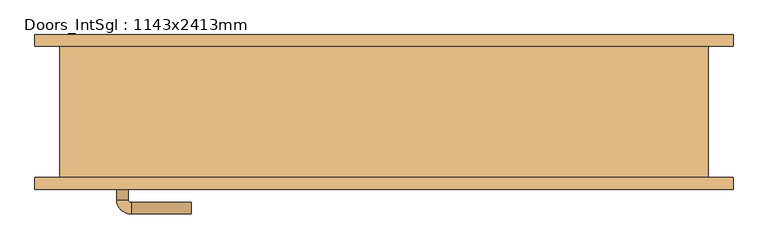
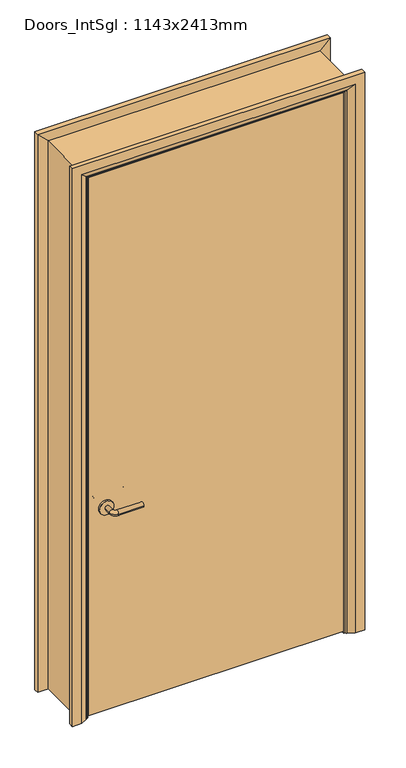
"""IFC4 building model written with IfcOpenShell, lengths in millimetres: door geometry, Doors_IntSgl : 1143x2413mm."""

from ifc_helpers import new_model, si_unit, point, frame, frame_2d, origin, place, context, project, spatial, polyline, circle_curve, ellipse_curve, trimmed, segment, composite_curve, outline, extrude, faceted_brep, source, transform, mapped, element, save
from ifc_brep_helpers import plane_surface, cylinder_surface, revolved_surface, advanced_brep


def doors_intsgl_1143x2413mm_ac4b68bc(model_context):
    return source(origin(), model_context, "Body", "SolidModel", [
        advanced_brep(
        [(-464.5, -68.3, 900.0), (-444.5, -68.3, 900.0), (-464.5, -38.3, 900.0), (-444.5, -38.3, 900.0), (-439.5, -33.3, 900.0), (-439.5, -13.3, 900.0), (-334.5, -13.3, 900.0), (-334.5, -33.3, 900.0)],
        [
            (0, 1, circle_curve(frame((-454.5, -68.3, 900.0), z_axis=(0.0, -1.0, 0.0), x_axis=(1.0, 0.0, 0.0)), 10.0)),
            (1, 0, circle_curve(frame((-454.5, -68.3, 900.0), z_axis=(0.0, -1.0, 0.0), x_axis=(1.0, 0.0, 0.0)), 10.0)),
            (0, 2),
            (2, 3, circle_curve(frame((-454.5, -38.3, 900.0), z_axis=(0.0, -1.0, 0.0), x_axis=(1.0, 0.0, 0.0)), 10.0)),
            (3, 1),
            (3, 2, circle_curve(frame((-454.5, -38.3, 900.0), z_axis=(0.0, -1.0, 0.0), x_axis=(1.0, 0.0, 0.0)), 10.0)),
            (4, 3, circle_curve(frame((-439.5, -38.3, 900.0), z_axis=(0.0, 0.0, 1.0), x_axis=(-1.0, 0.0, 0.0)), 5.0)),
            (2, 5, circle_curve(frame((-439.5, -38.3, 900.0), z_axis=(0.0, 0.0, -1.0), x_axis=(-1.0, 0.0, 0.0)), 25.0)),
            (5, 4, circle_curve(frame((-439.5, -23.3, 900.0), z_axis=(-1.0, 0.0, 0.0), x_axis=(0.0, -1.0, 0.0)), 10.0)),
            (4, 5, circle_curve(frame((-439.5, -23.3, 900.0), z_axis=(-1.0, 0.0, 0.0), x_axis=(0.0, -1.0, 0.0)), 10.0)),
            (6, 7, circle_curve(frame((-334.5, -23.3, 900.0), z_axis=(1.0, 0.0, 0.0), x_axis=(0.0, -1.0, 0.0)), 10.0)),
            (7, 6, circle_curve(frame((-334.5, -23.3, 900.0), z_axis=(1.0, 0.0, 0.0), x_axis=(0.0, -1.0, 0.0)), 10.0)),
            (5, 6),
            (7, 4),
        ],
        [
            plane_surface(frame((-454.5, -68.3, 900.0), z_axis=(0.0, -1.0, 0.0), x_axis=(0.0, 0.0, 1.0))),
            cylinder_surface(frame((-454.5, -68.3, 900.0), z_axis=(0.0, -1.0, 0.0), x_axis=(1.0, 0.0, 0.0)), 10.0),
            revolved_surface(trimmed(ellipse_curve(frame((-454.5, -38.3, 900.0), z_axis=(0.0, -1.0, 0.0), x_axis=(1.0, 0.0, 0.0)), 10.0, 10.0), [point((-464.5, -38.3, 900.0))], [point((-444.5, -38.3, 900.0))], True, "CARTESIAN"), (-439.5, -38.3, 900.0), (0.0, 0.0, -1.0)),
            revolved_surface(trimmed(ellipse_curve(frame((-454.5, -38.3, 900.0), z_axis=(0.0, -1.0, 0.0), x_axis=(1.0, 0.0, 0.0)), 10.0, 10.0), [point((-444.5, -38.3, 900.0))], [point((-464.5, -38.3, 900.0))], True, "CARTESIAN"), (-439.5, -38.3, 900.0), (0.0, 0.0, -1.0)),
            plane_surface(frame((-334.5, -23.3, 900.0), z_axis=(1.0, 0.0, 0.0), x_axis=(0.0, 0.0, 1.0))),
            cylinder_surface(frame((-439.5, -23.3, 900.0), z_axis=(-1.0, 0.0, 0.0), x_axis=(0.0, -1.0, 0.0)), 10.0),
        ],
        [
            (0, [[1, 2]]),
            (1, [[-1, 3, 4, 5]]),
            (1, [[-2, -5, 6, -3]]),
            (2, [[7, -4, 8, 9]]),
            (3, [[-8, -6, -7, 10]]),
            (4, [[11, 12]]),
            (5, [[-9, 13, -12, 14]]),
            (5, [[-10, -14, -11, -13]]),
        ],
    ),
        extrude(outline(composite_curve([segment(trimmed(circle_curve(frame_2d((900.0, -457.0)), 30.0), [point((900.0, -487.0))], [point((900.0, -427.0))], False, "CARTESIAN"), True, "CONTINUOUS"), segment(trimmed(circle_curve(frame_2d((900.0, -457.0)), 30.0), [point((900.0, -427.0))], [point((900.0, -487.0))], False, "CARTESIAN"), True, "CONTINUOUS")], self_intersect=False)), frame((0.0, -76.3, 0.0), z_axis=(0.0, 1.0, 0.0), x_axis=(0.0, 0.0, 1.0)), (0.0, 0.0, 1.0), 8.0),
        advanced_brep(
        [(-464.5, -122.3, 900.0), (-444.5, -122.3, 900.0), (-444.5, -152.3, 900.0), (-464.5, -152.3, 900.0), (-439.5, -157.3, 900.0), (-439.5, -177.3, 900.0), (-334.5, -177.3, 900.0), (-334.5, -157.3, 900.0)],
        [
            (0, 1, circle_curve(frame((-454.5, -122.3, 900.0), z_axis=(0.0, 1.0, 0.0), x_axis=(1.0, 0.0, 0.0)), 10.0)),
            (1, 0, circle_curve(frame((-454.5, -122.3, 900.0), z_axis=(0.0, 1.0, 0.0), x_axis=(1.0, 0.0, 0.0)), 10.0)),
            (1, 2),
            (2, 3, circle_curve(frame((-454.5, -152.3, 900.0), z_axis=(0.0, 1.0, 0.0), x_axis=(1.0, 0.0, 0.0)), 10.0)),
            (3, 0),
            (3, 2, circle_curve(frame((-454.5, -152.3, 900.0), z_axis=(0.0, 1.0, 0.0), x_axis=(1.0, 0.0, 0.0)), 10.0)),
            (4, 5, circle_curve(frame((-439.5, -167.3, 900.0), z_axis=(-1.0, 0.0, 0.0), x_axis=(0.0, 1.0, 0.0)), 10.0)),
            (5, 3, circle_curve(frame((-439.5, -152.3, 900.0), z_axis=(0.0, 0.0, -1.0), x_axis=(-1.0, 0.0, 0.0)), 25.0)),
            (2, 4, circle_curve(frame((-439.5, -152.3, 900.0), z_axis=(0.0, 0.0, 1.0), x_axis=(-1.0, 0.0, 0.0)), 5.0)),
            (5, 4, circle_curve(frame((-439.5, -167.3, 900.0), z_axis=(-1.0, 0.0, 0.0), x_axis=(0.0, 1.0, 0.0)), 10.0)),
            (6, 7, circle_curve(frame((-334.5, -167.3, 900.0), z_axis=(1.0, 0.0, 0.0), x_axis=(0.0, 1.0, 0.0)), 10.0)),
            (7, 6, circle_curve(frame((-334.5, -167.3, 900.0), z_axis=(1.0, 0.0, 0.0), x_axis=(0.0, 1.0, 0.0)), 10.0)),
            (4, 7),
            (6, 5),
        ],
        [
            plane_surface(frame((-454.5, -122.3, 900.0), z_axis=(0.0, 1.0, 0.0), x_axis=(0.0, 0.0, 1.0))),
            cylinder_surface(frame((-454.5, -122.3, 900.0), z_axis=(0.0, 1.0, 0.0), x_axis=(1.0, 0.0, 0.0)), 10.0),
            revolved_surface(trimmed(ellipse_curve(frame((-454.5, -152.3, 900.0), z_axis=(0.0, -1.0, 0.0), x_axis=(1.0, 0.0, 0.0)), 10.0, 10.0), [point((-464.5, -152.3, 900.0))], [point((-444.5, -152.3, 900.0))], True, "CARTESIAN"), (-439.5, -152.3, 900.0), (0.0, 0.0, -1.0)),
            revolved_surface(trimmed(ellipse_curve(frame((-454.5, -152.3, 900.0), z_axis=(0.0, -1.0, 0.0), x_axis=(1.0, 0.0, 0.0)), 10.0, 10.0), [point((-444.5, -152.3, 900.0))], [point((-464.5, -152.3, 900.0))], True, "CARTESIAN"), (-439.5, -152.3, 900.0), (0.0, 0.0, -1.0)),
            plane_surface(frame((-334.5, -167.3, 900.0), z_axis=(1.0, 0.0, 0.0), x_axis=(0.0, 0.0, 1.0))),
            cylinder_surface(frame((-439.5, -167.3, 900.0), z_axis=(-1.0, 0.0, 0.0), x_axis=(0.0, 1.0, 0.0)), 10.0),
        ],
        [
            (0, [[1, 2]]),
            (1, [[3, 4, 5, -2]]),
            (1, [[-5, 6, -3, -1]]),
            (2, [[7, 8, -4, 9]]),
            (3, [[10, -9, -6, -8]]),
            (4, [[11, 12]]),
            (5, [[13, -11, 14, -7]]),
            (5, [[-14, -12, -13, -10]]),
        ],
    ),
        extrude(outline(composite_curve([segment(trimmed(circle_curve(frame_2d((900.0, -457.0)), 30.0), [point((900.0, -487.0))], [point((900.0, -427.0))], False, "CARTESIAN"), True, "CONTINUOUS"), segment(trimmed(circle_curve(frame_2d((900.0, -457.0)), 30.0), [point((900.0, -427.0))], [point((900.0, -487.0))], False, "CARTESIAN"), True, "CONTINUOUS")], self_intersect=False)), frame((0.0, -122.3, 0.0), z_axis=(0.0, 1.0, 0.0), x_axis=(0.0, 0.0, 1.0)), (0.0, 0.0, 1.0), 8.0),
        extrude(outline(polyline([(529.5, -76.3), (529.5, -114.3), (-529.5, -114.3), (-529.5, -76.3), (529.5, -76.3)])), frame((0.0, 0.0, 8.0), z_axis=(0.0, 0.0, 1.0), x_axis=(1.0, 0.0, 0.0)), (0.0, 0.0, 1.0), 2363.0),
        advanced_brep(
        [(606.5, -134.3, 0.0), (566.5, -134.3, 0.0), (540.5, -120.3, 0.0), (536.5, -114.3, 0.0), (606.5, -114.3, 0.0), (606.5, -114.3, 2448.0), (606.5, -134.3, 2448.0), (536.5, -114.3, 2378.0), (-536.5, -114.3, 2378.0), (-536.5, -114.3, 0.0), (-606.5, -114.3, 0.0), (-606.5, -114.3, 2448.0), (540.5, -120.3, 2382.0), (566.5, -134.3, 2408.0), (-606.5, -134.3, 2448.0), (-606.5, -134.3, 0.0), (-566.5, -134.3, 0.0), (-566.5, -134.3, 2408.0), (-540.5, -120.3, 2382.0), (-540.5, -120.3, 0.0)],
        [
            (0, 1),
            (1, 2),
            (2, 3, circle_curve(frame((544.5, -113.3, 0.0), z_axis=(0.0, 0.0, -1.0), x_axis=(1.0, 0.0, 0.0)), 8.0622577)),
            (3, 4),
            (4, 0),
            (4, 5),
            (5, 6),
            (6, 0),
            (3, 7),
            (7, 8),
            (8, 9),
            (9, 10),
            (10, 11),
            (11, 5),
            (2, 12),
            (12, 7, ellipse_curve(frame((544.5, -113.3, 2386.0), z_axis=(0.7071067811865475, 0.0, -0.7071067811865475), x_axis=(-0.7071067811865474, 0.0, -0.7071067811865476)), 11.4017543, 8.0622577)),
            (1, 13),
            (13, 12),
            (6, 14),
            (14, 15),
            (15, 16),
            (16, 17),
            (17, 13),
            (11, 14),
            (12, 18),
            (18, 8, ellipse_curve(frame((-544.5, -113.3, 2386.0), z_axis=(0.7071067811865475, 0.0, 0.7071067811865475), x_axis=(0.7071067811865476, 0.0, -0.7071067811865474)), 11.4017543, 8.0622577)),
            (17, 18),
            (15, 10),
            (9, 19, circle_curve(frame((-544.5, -113.3, 0.0), z_axis=(0.0, 0.0, -1.0), x_axis=(-1.0, 0.0, 0.0)), 8.0622577)),
            (19, 16),
            (18, 19),
        ],
        [
            plane_surface(frame((536.5, -114.3, 0.0), z_axis=(0.0, 0.0, -1.0), x_axis=(0.0, 1.0, 0.0))),
            plane_surface(frame((606.5, -134.3, 0.0), z_axis=(1.0, 0.0, 0.0), x_axis=(0.0, 0.0, 1.0))),
            plane_surface(frame((606.5, -114.3, 0.0), z_axis=(0.0, 1.0, 0.0), x_axis=(0.0, 0.0, 1.0))),
            cylinder_surface(frame((544.5, -113.3, 0.0), z_axis=(0.0, 0.0, -1.0), x_axis=(1.0, 0.0, 0.0)), 8.0622577),
            plane_surface(frame((540.5, -120.3, 0.0), z_axis=(-0.4740998230350126, -0.880471099922178, 0.0), x_axis=(0.0, 0.0, 1.0))),
            plane_surface(frame((566.5, -134.3, 0.0), z_axis=(0.0, -1.0, 0.0), x_axis=(0.0, 0.0, 1.0))),
            plane_surface(frame((606.5, -134.3, 2448.0), z_axis=(0.0, 0.0, 1.0), x_axis=(-1.0, 0.0, 0.0))),
            cylinder_surface(frame((536.5, -113.3, 2386.0), z_axis=(1.0, 0.0, 0.0), x_axis=(0.0, 0.0, 1.0)), 8.0622577),
            plane_surface(frame((540.5, -120.3, 2382.0), z_axis=(0.0, -0.8804710999221764, -0.4740998230350154), x_axis=(-1.0, 0.0, 0.0))),
            plane_surface(frame((-536.5, -114.3, 0.0), z_axis=(0.0, 0.0, -1.0), x_axis=(0.0, 1.0, 0.0))),
            plane_surface(frame((-606.5, -134.3, 2448.0), z_axis=(-1.0, 0.0, 0.0), x_axis=(0.0, 0.0, -1.0))),
            cylinder_surface(frame((-544.5, -113.3, 2378.0), z_axis=(0.0, 0.0, 1.0), x_axis=(-1.0, 0.0, 0.0)), 8.0622577),
            plane_surface(frame((-540.5, -120.3, 2382.0), z_axis=(0.47409982303501824, -0.8804710999221749, 0.0), x_axis=(0.0, 0.0, -1.0))),
        ],
        [
            (0, [[1, 2, 3, 4, 5]]),
            (1, [[6, 7, 8, -5]]),
            (2, [[9, 10, 11, 12, 13, 14, -6, -4]]),
            (3, [[15, 16, -9, -3]]),
            (4, [[17, 18, -15, -2]]),
            (5, [[-8, 19, 20, 21, 22, 23, -17, -1]]),
            (6, [[-14, 24, -19, -7]]),
            (7, [[25, 26, -10, -16]]),
            (8, [[-23, 27, -25, -18]]),
            (9, [[28, -12, 29, 30, -21]]),
            (10, [[-13, -28, -20, -24]]),
            (11, [[31, -29, -11, -26]]),
            (12, [[-22, -30, -31, -27]]),
        ],
    ),
        extrude(outline(polyline([(0.0, -512.5), (2354.0, -512.5), (2354.0, 512.5), (0.0, 512.5), (0.0, 531.5), (2373.0, 531.5), (2373.0, -531.5), (0.0, -531.5), (0.0, -512.5)])), frame((0.0, -74.3, 0.0), z_axis=(0.0, 1.0, 0.0), x_axis=(0.0, 0.0, 1.0)), (0.0, 0.0, 1.0), 32.0),
        advanced_brep(
        [(-606.5, 134.3, 0.0), (-566.5, 134.3, 0.0), (-540.5, 120.3, 0.0), (-536.5, 114.3, 0.0), (-606.5, 114.3, 0.0), (-606.5, 114.3, 2448.0), (-606.5, 134.3, 2448.0), (-536.5, 114.3, 2378.0), (-540.5, 120.3, 2382.0), (-566.5, 134.3, 2408.0), (606.5, 114.3, 2448.0), (606.5, 134.3, 2448.0), (536.5, 114.3, 2378.0), (540.5, 120.3, 2382.0), (566.5, 134.3, 2408.0), (606.5, 134.3, 0.0), (606.5, 114.3, 0.0), (536.5, 114.3, 0.0), (540.5, 120.3, 0.0), (566.5, 134.3, 0.0)],
        [
            (0, 1),
            (1, 2),
            (2, 3, circle_curve(frame((-544.5, 113.3, 0.0), z_axis=(0.0, 0.0, -1.0), x_axis=(-1.0, 0.0, 0.0)), 8.0622577)),
            (3, 4),
            (4, 0),
            (4, 5),
            (5, 6),
            (6, 0),
            (3, 7),
            (7, 5),
            (2, 8),
            (8, 7, ellipse_curve(frame((-544.5, 113.3, 2386.0), z_axis=(-0.7071067811865475, 0.0, -0.7071067811865475), x_axis=(0.7071067811865474, 0.0, -0.7071067811865476)), 11.4017543, 8.0622577)),
            (1, 9),
            (9, 8),
            (6, 9),
            (5, 10),
            (10, 11),
            (11, 6),
            (7, 12),
            (12, 10),
            (8, 13),
            (13, 12, ellipse_curve(frame((544.5, 113.3, 2386.0), z_axis=(-0.7071067811865475, 0.0, 0.7071067811865475), x_axis=(-0.7071067811865476, 0.0, -0.7071067811865474)), 11.4017543, 8.0622577)),
            (9, 14),
            (14, 13),
            (11, 14),
            (15, 16),
            (16, 17),
            (17, 18, circle_curve(frame((544.5, 113.3, 0.0), z_axis=(0.0, 0.0, -1.0), x_axis=(1.0, 0.0, 0.0)), 8.0622577)),
            (18, 19),
            (19, 15),
            (10, 16),
            (15, 11),
            (12, 17),
            (13, 18),
            (14, 19),
        ],
        [
            plane_surface(frame((-536.5, 187.1010989, 0.0), z_axis=(0.0, 0.0, -1.0), x_axis=(1.0, 0.0, 0.0))),
            plane_surface(frame((-606.5, 134.3, 0.0), z_axis=(-1.0, 0.0, 0.0), x_axis=(0.0, 0.0, 1.0))),
            plane_surface(frame((-606.5, 114.3, 0.0), z_axis=(0.0, -1.0, 0.0), x_axis=(0.0, 0.0, 1.0))),
            cylinder_surface(frame((-544.5, 113.3, 0.0), z_axis=(0.0, 0.0, -1.0), x_axis=(-1.0, 0.0, 0.0)), 8.0622577),
            plane_surface(frame((-540.5, 120.3, 0.0), z_axis=(0.4740998230350183, 0.8804710999221749, 0.0), x_axis=(0.0, 0.0, 1.0))),
            plane_surface(frame((-566.5, 134.3, 0.0), z_axis=(0.0, 1.0, 0.0), x_axis=(0.0, 0.0, 1.0))),
            plane_surface(frame((-606.5, 134.3, 2448.0), z_axis=(0.0, 0.0, 1.0), x_axis=(1.0, 0.0, 0.0))),
            plane_surface(frame((-606.5, 114.3, 2448.0), z_axis=(0.0, -1.0, 0.0), x_axis=(1.0, 0.0, 0.0))),
            cylinder_surface(frame((-536.5, 113.3, 2386.0), z_axis=(-1.0, 0.0, 0.0), x_axis=(0.0, 0.0, 1.0)), 8.0622577),
            plane_surface(frame((-540.5, 120.3, 2382.0), z_axis=(0.0, 0.8804710999221749, -0.4740998230350183), x_axis=(1.0, 0.0, 0.0))),
            plane_surface(frame((-566.5, 134.3, 2408.0), z_axis=(0.0, 1.0, 0.0), x_axis=(1.0, 0.0, 0.0))),
            plane_surface(frame((536.5, 187.1010989, 0.0), z_axis=(0.0, 0.0, -1.0), x_axis=(-1.0, 0.0, 0.0))),
            plane_surface(frame((606.5, 134.3, 2448.0), z_axis=(1.0, 0.0, 0.0), x_axis=(0.0, 0.0, -1.0))),
            plane_surface(frame((606.5, 114.3, 2448.0), z_axis=(0.0, -1.0, 0.0), x_axis=(0.0, 0.0, -1.0))),
            cylinder_surface(frame((544.5, 113.3, 2378.0), z_axis=(0.0, 0.0, 1.0), x_axis=(1.0, 0.0, 0.0)), 8.0622577),
            plane_surface(frame((540.5, 120.3, 2382.0), z_axis=(-0.4740998230350183, 0.8804710999221749, 0.0), x_axis=(0.0, 0.0, -1.0))),
            plane_surface(frame((566.5, 134.3, 2408.0), z_axis=(0.0, 1.0, 0.0), x_axis=(0.0, 0.0, -1.0))),
        ],
        [
            (0, [[1, 2, 3, 4, 5]]),
            (1, [[6, 7, 8, -5]]),
            (2, [[9, 10, -6, -4]]),
            (3, [[11, 12, -9, -3]]),
            (4, [[13, 14, -11, -2]]),
            (5, [[-8, 15, -13, -1]]),
            (6, [[16, 17, 18, -7]]),
            (7, [[19, 20, -16, -10]]),
            (8, [[21, 22, -19, -12]]),
            (9, [[23, 24, -21, -14]]),
            (10, [[-18, 25, -23, -15]]),
            (11, [[26, 27, 28, 29, 30]]),
            (12, [[31, -26, 32, -17]]),
            (13, [[33, -27, -31, -20]]),
            (14, [[34, -28, -33, -22]]),
            (15, [[35, -29, -34, -24]]),
            (16, [[-32, -30, -35, -25]]),
        ],
    ),
        faceted_brep([(-531.5, -114.3, 0.0), (-563.5, -114.3, 0.0), (-563.5, 114.3, 0.0), (-531.5, 114.3, 0.0), (-531.5, 114.3, 2373.0), (-531.5, -114.3, 2373.0), (-563.5, 114.3, 2405.0), (-563.5, -114.3, 2405.0), (531.5, 114.3, 2373.0), (531.5, -114.3, 2373.0), (563.5, 114.3, 2405.0), (563.5, -114.3, 2405.0), (531.5, -114.3, 0.0), (531.5, 114.3, 0.0), (563.5, 114.3, 0.0), (563.5, -114.3, 0.0)], [[[0, 1, 2, 3]], [[3, 4, 5, 0]], [[2, 6, 4, 3]], [[1, 7, 6, 2]], [[0, 5, 7, 1]], [[4, 8, 9, 5]], [[6, 10, 8, 4]], [[7, 11, 10, 6]], [[5, 9, 11, 7]], [[12, 13, 14, 15]], [[8, 13, 12, 9]], [[10, 14, 13, 8]], [[11, 15, 14, 10]], [[9, 12, 15, 11]]]),
    ])


if __name__ == "__main__":
    model = new_model("IFC4")
    model_context = context("Model", 3, world=origin())
    ifc_project = project(units=[si_unit("LENGTHUNIT", "METRE", prefix="MILLI")], contexts=[model_context])
    site = spatial("IfcSite", under=ifc_project)
    building = spatial("IfcBuilding", under=site)
    placement = place(None, origin())
    doors_intsgl_1143x2413mm_shape = doors_intsgl_1143x2413mm_ac4b68bc(model_context)
    element("IfcDoor", 1, ObjectType="Doors_IntSgl : 1143x2413mm", at=placement, inside=building, context=model_context, shape_type="MappedRepresentation", body=[
        mapped(doors_intsgl_1143x2413mm_shape, transform((0.0, 0.0, 0.0), x_axis=(1.0, 0.0, 0.0), y_axis=(0.0, 1.0, 0.0), z_axis=(0.0, 0.0, 1.0))),
    ])
    save(model, "model.ifc")

# Revit data of these elements
# Type "Doors_IntSgl : 1143x2413mm"
#   Construction Type Id = "MDOOR"
#   Type Mark = "43"
#   Type Comments = "Internal Single"
#   Operation = "SingleSwingRight"
#   Manufacturer = "Revit"
#   Keynote = "L20"
#   Description = "Internal Single Door"
#   Analytic Construction = "Metal"
#   UnderCut = 0' - 0.31496"
#   Tolerance = 0' - 0.07874"
#   Thickness = 0' - 1.49606"
#   Thermal Resistance (R) = 0.270117 (m²·K)/W
#   Structural Tolerance = 0' - 0.31496"
#   StopDepth = 0' - 1.25984"
#   Stop Thickness = 0' - 0.74803"
#   Rough Width = 3' - 9"
#   Rough Height = 7' - 11"
#   Height to Top Lock Rail = 3' - 3.37008"
#   Heat Transfer Coefficient (U) = 3.7021 W/(m²·K)
#   Handle Z Distance = 2' - 11.43307"
#   Handle X Distance = 0' - 2.95276"
#   Frame Thickness = 0' - 1.25984"
#   Door Panel Width = 3' - 5.69291"
#   Door Panel Thickness = 0' - 1.49606"
#   Door Panel Offset = 0' - 0"
#   Height = 7' - 11"
#   Width = 3' - 9"
#   Door Panel Height = 7' - 9.0315"
#   Architrave Setback = 0' - 0.19685"
#   Define Thermal Properties by = 1
#   Vis - Ironmongery = yes
#   Material Ironmongery = Door - Handle
#   Material Frame = Door - Frame/Mullion (1)
#   Material Door = Door - Panel
#   Material Architrave = Door - Architrave
#   Visual Light Transmittance = 0
#   Solar Heat Gain Coefficient = 0
#   Function = (empty or 0)
#   Wall Closure = (empty or 0)
# Element 1 (IfcDoor, "Doors_IntSgl : 1143x2413mm")
#   Materials on its faces: "Door - Architrave", "Door - Handle", "Door - Frame/Mullion (1)", "Door - Panel"
# Materials
#   "Door - Handle": colour RGB 0 0 0, transparency 0, Keynote = "P21", Cost = 0
#   "Door - Frame/Mullion (1)": class "Wood", colour RGB 212 179 113, transparency 0, Keynote = "L20", Cost = 0
#   "Door - Panel": class "Wood", colour RGB 210 159 95, transparency 0, Keynote = "L20", Cost = 0
#   "Door - Architrave": class "Wood", colour RGB 154 90 5, transparency 0, Keynote = "P20", Cost = 0
